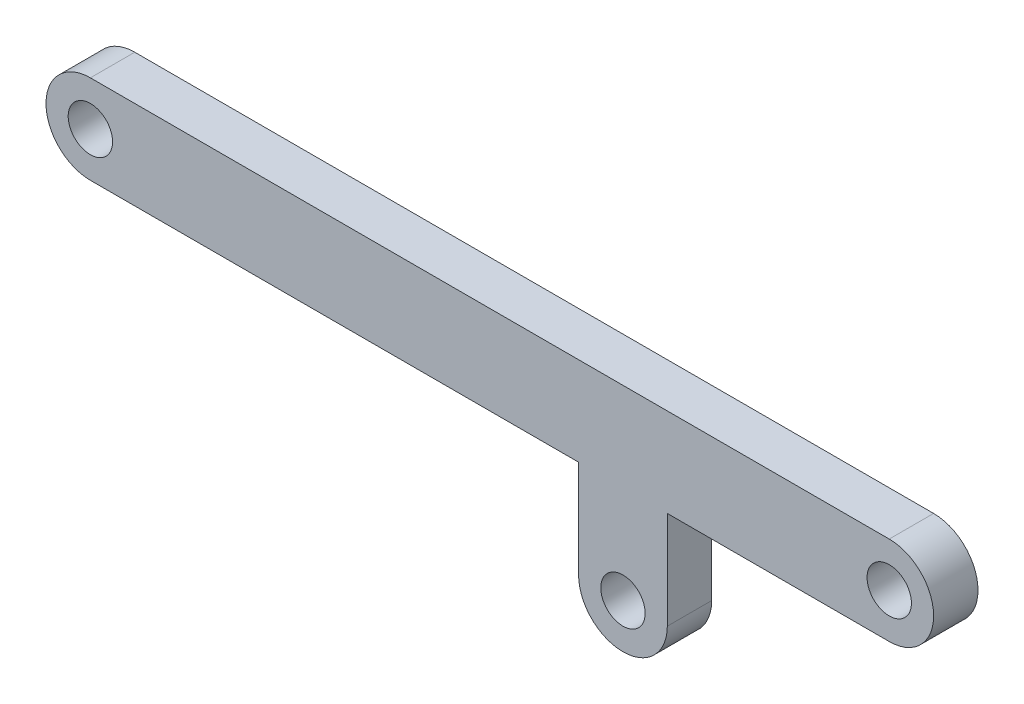
from build123d import *

# Parameters (mm, degrees)
LINK_PLATE_PROFILE_R = 2.5
LINK_PLATE_PROFILE_W = 10
LINK_PLATE_PROFILE_H = 10
LINK_PLATE_5MM_DEPTH = 2.5


with BuildPart() as part:
    # Link Plate Profile → Link Plate 5mm (new, symmetric)
    # profile 1 of 4: a face of its own
    with BuildSketch(Plane.XY):
        with BuildLine():
            Line((-45, -5), (10, -5))
            Line((10, -5), (10, 5))
            Line((10, 5), (-45, 5))
            ThreePointArc((-45, 5), (-50, 0), (-45, -5))
        make_face()
        with Locations((-45, 0)):
            Circle(LINK_PLATE_PROFILE_R, mode=Mode.SUBTRACT)
    # profile 2 of 4: a face of its own
    with BuildSketch(Plane.XY):
        with Locations((15, 0)):
            Rectangle(LINK_PLATE_PROFILE_W, LINK_PLATE_PROFILE_H)
    # profile 3 of 4: a face of its own
    with BuildSketch(Plane.XY):
        with BuildLine():
            Line((20, -5), (45, -5))
            ThreePointArc((45, -5), (50, 0), (45, 5))
            Line((45, 5), (20, 5))
            Line((20, 5), (20, -5))
        make_face()
        with Locations((45, 0)):
            Circle(LINK_PLATE_PROFILE_R, mode=Mode.SUBTRACT)
    # profile 4 of 4: a face of its own
    with BuildSketch(Plane.XY):
        with BuildLine():
            Line((20, -16), (20, -5))
            Line((20, -5), (10, -5))
            Line((10, -5), (10, -16))
            ThreePointArc((10, -16), (15, -21), (20, -16))
        make_face()
        with Locations((15, -16)):
            Circle(LINK_PLATE_PROFILE_R, mode=Mode.SUBTRACT)
    extrude(amount=LINK_PLATE_5MM_DEPTH, both=True)


solid = part.part
